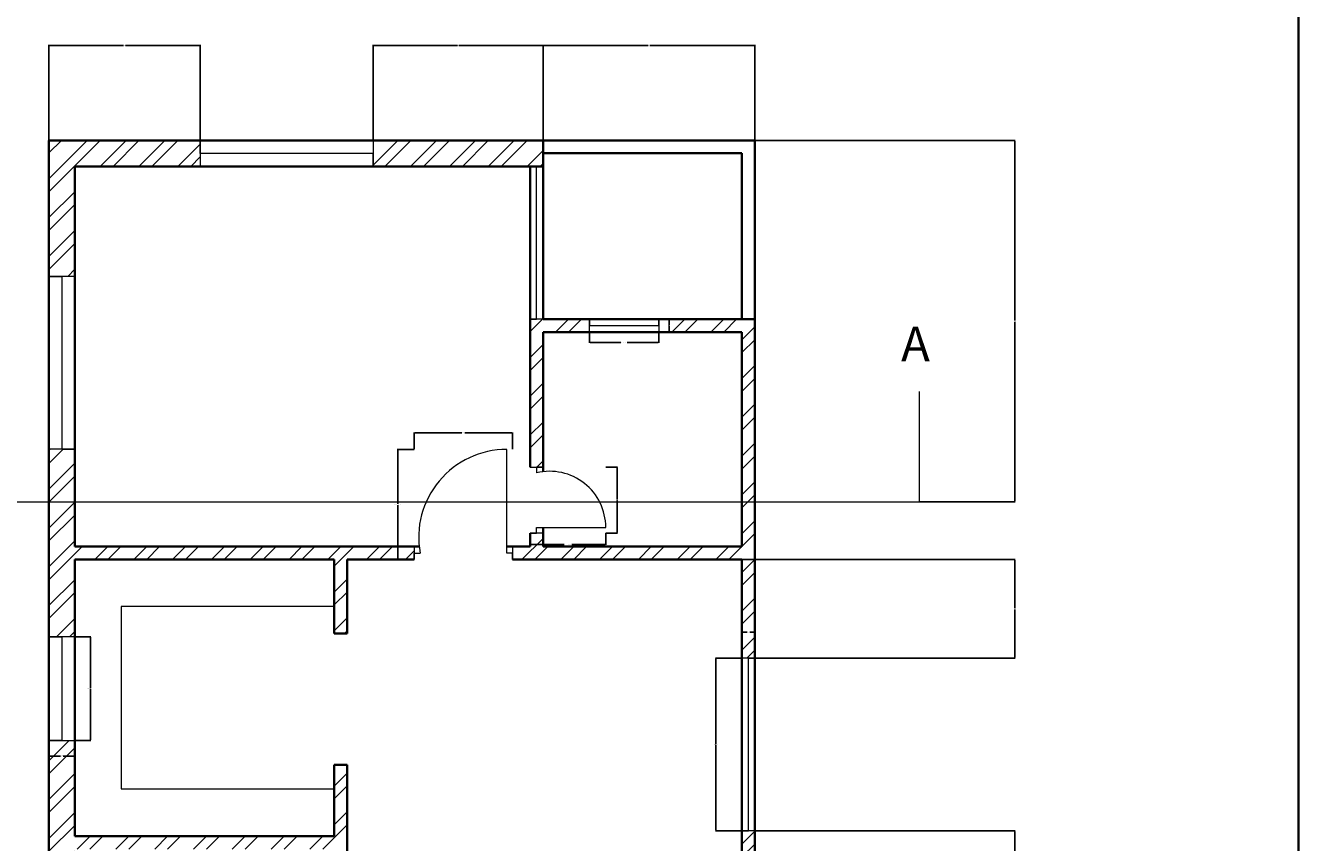
# Model space of a CAD drawing. Units: inches. Extents: x 1850 to 3445, y 1558 to 2756.
# Tile 12 of 13: x 3003 to 3445, y 1972 to 2256. Entities that reach past the tile are written whole.
import ezdxf

# ---------------------------------------------------------------- set-up
doc = ezdxf.new("R2010")
doc.units = ezdxf.units.IN
for name, color, linetype, lineweight in [('A-ANNO-DIMS', 2, 'Continuous', 18), ('A-ANNO-SYMB', 2, 'Continuous', 18), ('A-ANNO-TTLB', 7, 'Continuous', 35), ('A-DOOR', 3, 'Continuous', 18), ('A-FLOR-CASE', 8, 'Continuous', 18), ('A-GLAZ', 4, 'Continuous', 18), ('A-WALL', 7, 'Continuous', 35), ('A-WALL-PATT', 252, 'Continuous', 13)]:
    doc.layers.add(name, color=color, linetype=linetype, lineweight=lineweight)
doc.styles.get("Standard").update_dxf_attribs({"font": 'arial.ttf'})
doc.dimstyles.get("Standard").update_dxf_attribs({"dimtxt": 0.18, "dimasz": 0.18, "dimexe": 0.18, "dimexo": 0.0625, "dimgap": 0.09, "dimtad": 0, "dimtih": 1, "dimtoh": 1, "dimdec": 4, "dimzin": 0, "dimdsep": 46, "dimtxsty": 'Standard', "dimcen": 0.09, "dimadec": 0, "dimazin": 0, "dimtfac": 1, "dimtdec": 4, "dimtofl": 0, "dimtmove": 0, "dimatfit": 3, "dimfxl": 1, "dimtolj": 1, "dimtzin": 0, "dimarcsym": 0})
pattern_1 = [(45, (660.551, 0), (-6.735192, 6.735192), []), (45, (665.041, 0), (-6.735192, 6.735192), [])]

# ---------------------------------------------------------------- blocks, each defined once
blk = doc.blocks.new('WIN-60-W9')
for p, q in [((0, 9), (0, 0)), ((60, 4.5), (60, 9)), ((60, 9), (60, 0)), ((0, 0), (0, 4.5)), ((0, 4.5), (60, 4.5))]:
    blk.add_line(p, q)
blk = doc.blocks.new('WIN-36-W9-ALT')
for p, q in [((9, 36), (0, 36)), ((0, 36), (4.5, 36)), ((4.5, 36), (4.5, 0)), ((4.5, 0), (0, 0)), ((0, 0), (9, 0))]:
    blk.add_line(p, q)
blk = doc.blocks.new('WIN-60-W4_5')
for p, q in [((0, 60), (4.5, 60)), ((4.5, 60), (2.25, 60)), ((2.25, 60), (2.25, 0)), ((2.25, 0), (0, 0)), ((0, 0), (4.5, 0))]:
    blk.add_line(p, q)
blk = doc.blocks.new('WIN-24-W4_5')
for p, q in [((0, 0), (0, 4.5)), ((0, 4.5), (0, 2.25)), ((24, 2.25), (24, 4.5)), ((24, 4.5), (24, 0)), ((0, 2.25), (24, 2.25))]:
    blk.add_line(p, q)
blk = doc.blocks.new('DOOR-BATH-REAR-UPPER')
for p, q in [((0, 22.93), (4.5, 22.93)), ((4.5, 22.93), (2.25, 22.93)), ((2.25, 22.93), (2.25, 20.93)), ((2.25, 0), (2.25, 2)), ((2.25, 2), (26.25, 2)), ((4.5, 0), (0, 0)), ((0, 0), (2.25, 0))]:
    blk.add_line(p, q)
blk.add_arc((6.78, 2), 19.47, 0, 103.4712)
blk = doc.blocks.new('DOOR-BED-UPPER')
for p, q in [((32.07, 2.25), (32.07, 38.25)), ((0, 4.5), (0, 0)), ((34.07, 4.5), (34.07, 0)), ((0, 0), (0, 2.25)), ((0, 2.25), (2, 2.25)), ((34.07, 2.25), (32.07, 2.25)), ((34.07, 0), (34.07, 2.25))]:
    blk.add_line(p, q)
blk.add_arc((32.07, 7.69), 30.56, 90, 190.2532)
blk = doc.blocks.new('COUNTER-U-UPPER')
for p, q in [((73.88, 63.24), (0, 63.24)), ((0, 63.24), (0, 0)), ((0, 0), (73.88, 0))]:
    blk.add_line(p, q)
blk = doc.blocks.new('*D30')
at = {"layer": 'A-ANNO-DIMS', "color": 0, "lineweight": -2, "transparency": 16777216}
for p, q in [((3252.04, 2036.5), (3242.93, 2036.5)), ((3243.11, 2036.32), (3243.11, 2006.68)), ((3243.11, 1976.68), (3243.11, 2006.31)), ((3252.04, 1976.5), (3242.93, 1976.5))]:
    blk.add_line(p, q, dxfattribs=at)
at = {"layer": 'A-ANNO-DIMS', "color": 0, "transparency": 16777216}
for points in [[(3243.08, 2036.32), (3243.14, 2036.32), (3243.11, 2036.5)], [(3243.08, 1976.68), (3243.14, 1976.68), (3243.11, 1976.5)]]:
    blk.add_solid(points, dxfattribs=at)
at = {"layer": 'Defpoints', "color": 0, "transparency": 16777216}
for p in [(3252.11, 2036.5), (3243.11, 1976.5), (3252.11, 1976.5)]:
    blk.add_point(p, dxfattribs=at)
at = {"layer": 'A-ANNO-DIMS', "color": 0, "transparency": 16777216, "insert": (3243.11, 2006.5), "char_height": 0.18, "attachment_point": 5}
blk.add_mtext('\\A1;WINDOW 60 TYP.', dxfattribs=at)
blk = doc.blocks.new('*D31')
at = {"layer": 'A-ANNO-DIMS', "color": 0, "lineweight": -2, "transparency": 16777216}
for p, q in [((3252.11, 2036.56), (3252.11, 2045.68)), ((3256.61, 2036.56), (3256.61, 2045.68)), ((3252.29, 2045.5), (3253.9, 2045.5)), ((3256.43, 2045.5), (3254.81, 2045.5))]:
    blk.add_line(p, q, dxfattribs=at)
at = {"layer": 'A-ANNO-DIMS', "color": 0, "transparency": 16777216}
for points in [[(3252.29, 2045.53), (3252.29, 2045.47), (3252.11, 2045.5)], [(3256.43, 2045.53), (3256.43, 2045.47), (3256.61, 2045.5)]]:
    blk.add_solid(points, dxfattribs=at)
at = {"layer": 'Defpoints', "color": 0, "transparency": 16777216}
for p in [(3252.11, 2045.5), (3252.11, 2036.5), (3256.61, 2036.5)]:
    blk.add_point(p, dxfattribs=at)
at = {"layer": 'A-ANNO-DIMS', "color": 0, "transparency": 16777216, "insert": (3254.36, 2045.5), "char_height": 0.18, "attachment_point": 5}
blk.add_mtext('\\A1;5 TYP.', dxfattribs=at)
blk = doc.blocks.new('*D38')
at = {"layer": 'A-ANNO-DIMS', "color": 0, "lineweight": -2, "transparency": 16777216}
for p, q in [((3020.67, 2043.87), (3026.19, 2043.87)), ((3026.01, 2043.69), (3026.01, 2026.05)), ((3026.01, 2008.05), (3026.01, 2025.69)), ((3020.67, 2007.87), (3026.19, 2007.87))]:
    blk.add_line(p, q, dxfattribs=at)
at = {"layer": 'A-ANNO-DIMS', "color": 0, "transparency": 16777216}
for points in [[(3025.98, 2043.69), (3026.04, 2043.69), (3026.01, 2043.87)], [(3025.98, 2008.05), (3026.04, 2008.05), (3026.01, 2007.87)]]:
    blk.add_solid(points, dxfattribs=at)
at = {"layer": 'Defpoints', "color": 0, "transparency": 16777216}
for p in [(3020.61, 2043.87), (3026.01, 2043.87), (3020.61, 2007.87)]:
    blk.add_point(p, dxfattribs=at)
at = {"layer": 'A-ANNO-DIMS', "color": 0, "transparency": 16777216, "insert": (3026.01, 2025.87), "char_height": 0.18, "attachment_point": 5}
blk.add_mtext('\\A1;WINDOW 36 TYP.', dxfattribs=at)
blk = doc.blocks.new('*D39')
at = {"layer": 'A-ANNO-DIMS', "color": 0, "lineweight": -2, "transparency": 16777216}
for p, q in [((3011.61, 2007.81), (3011.61, 2002.29)), ((3020.61, 2007.81), (3020.61, 2002.29)), ((3011.79, 2002.47), (3015.65, 2002.47)), ((3020.43, 2002.47), (3016.56, 2002.47))]:
    blk.add_line(p, q, dxfattribs=at)
at = {"layer": 'A-ANNO-DIMS', "color": 0, "transparency": 16777216}
for points in [[(3011.79, 2002.5), (3011.79, 2002.44), (3011.61, 2002.47)], [(3020.43, 2002.5), (3020.43, 2002.44), (3020.61, 2002.47)]]:
    blk.add_solid(points, dxfattribs=at)
at = {"layer": 'Defpoints', "color": 0, "transparency": 16777216}
for p in [(3011.61, 2007.87), (3020.61, 2007.87), (3020.61, 2002.47)]:
    blk.add_point(p, dxfattribs=at)
at = {"layer": 'A-ANNO-DIMS', "color": 0, "transparency": 16777216, "insert": (3016.11, 2002.47), "char_height": 0.18, "attachment_point": 5}
blk.add_mtext('\\A1;9 TYP.', dxfattribs=at)
blk = doc.blocks.new('*D42')
at = {"layer": 'A-ANNO-DIMS', "color": 0, "lineweight": -2, "transparency": 16777216}
for p, q in [((3199.22, 2149.62), (3199.22, 2145.9)), ((3223.22, 2149.62), (3223.22, 2145.9)), ((3199.4, 2146.08), (3210.1, 2146.08)), ((3223.04, 2146.08), (3212.33, 2146.08))]:
    blk.add_line(p, q, dxfattribs=at)
at = {"layer": 'A-ANNO-DIMS', "color": 0, "transparency": 16777216}
for points in [[(3199.4, 2146.11), (3199.4, 2146.05), (3199.22, 2146.08)], [(3223.04, 2146.11), (3223.04, 2146.05), (3223.22, 2146.08)]]:
    blk.add_solid(points, dxfattribs=at)
at = {"layer": 'Defpoints', "color": 0, "transparency": 16777216}
for p in [(3199.22, 2149.68), (3223.22, 2149.68), (3223.22, 2146.08)]:
    blk.add_point(p, dxfattribs=at)
at = {"layer": 'A-ANNO-DIMS', "color": 0, "transparency": 16777216, "insert": (3211.22, 2146.08), "char_height": 0.18, "attachment_point": 5}
blk.add_mtext('\\A1;WINDOW 24 TYP.', dxfattribs=at)
blk = doc.blocks.new('*D43')
at = {"layer": 'A-ANNO-DIMS', "color": 0, "lineweight": -2, "transparency": 16777216}
for p, q in [((3223.28, 2154.18), (3227, 2154.18)), ((3226.82, 2154), (3226.82, 2152.12)), ((3226.82, 2149.86), (3226.82, 2151.75)), ((3223.28, 2149.68), (3227, 2149.68))]:
    blk.add_line(p, q, dxfattribs=at)
at = {"layer": 'A-ANNO-DIMS', "color": 0, "transparency": 16777216}
for points in [[(3226.79, 2154), (3226.85, 2154), (3226.82, 2154.18)], [(3226.79, 2149.86), (3226.85, 2149.86), (3226.82, 2149.68)]]:
    blk.add_solid(points, dxfattribs=at)
at = {"layer": 'Defpoints', "color": 0, "transparency": 16777216}
for p in [(3223.22, 2154.18), (3226.82, 2154.18), (3223.22, 2149.68)]:
    blk.add_point(p, dxfattribs=at)
at = {"layer": 'A-ANNO-DIMS', "color": 0, "transparency": 16777216, "insert": (3226.82, 2151.93), "char_height": 0.18, "attachment_point": 5}
blk.add_mtext('\\A1;5 TYP.', dxfattribs=at)
blk = doc.blocks.new('*D62')
at = {"layer": 'A-ANNO-DIMS', "color": 0, "lineweight": -2, "transparency": 16777216}
for p, q in [((3178.61, 2079.81), (3178.61, 2075.75)), ((3204.86, 2079.81), (3204.86, 2075.75)), ((3178.79, 2075.93), (3190.42, 2075.93)), ((3204.68, 2075.93), (3193.04, 2075.93))]:
    blk.add_line(p, q, dxfattribs=at)
at = {"layer": 'A-ANNO-DIMS', "color": 0, "transparency": 16777216}
for points in [[(3178.79, 2075.96), (3178.79, 2075.9), (3178.61, 2075.93)], [(3204.68, 2075.96), (3204.68, 2075.9), (3204.86, 2075.93)]]:
    blk.add_solid(points, dxfattribs=at)
at = {"layer": 'Defpoints', "color": 0, "transparency": 16777216}
for p in [(3178.61, 2079.87), (3204.86, 2079.87), (3204.86, 2075.93)]:
    blk.add_point(p, dxfattribs=at)
at = {"layer": 'A-ANNO-DIMS', "color": 0, "transparency": 16777216, "insert": (3191.73, 2075.93), "char_height": 0.18, "attachment_point": 5}
blk.add_mtext('\\A1;BATH DOOR 26 TYP.', dxfattribs=at)
blk = doc.blocks.new('*D63')
at = {"layer": 'A-ANNO-DIMS', "color": 0, "lineweight": -2, "transparency": 16777216}
for p, q in [((3204.92, 2102.8), (3208.97, 2102.8)), ((3208.79, 2102.62), (3208.79, 2091.52)), ((3208.79, 2080.05), (3208.79, 2091.15)), ((3204.92, 2079.87), (3208.97, 2079.87))]:
    blk.add_line(p, q, dxfattribs=at)
at = {"layer": 'A-ANNO-DIMS', "color": 0, "transparency": 16777216}
for points in [[(3208.76, 2102.62), (3208.82, 2102.62), (3208.79, 2102.8)], [(3208.76, 2080.05), (3208.82, 2080.05), (3208.79, 2079.87)]]:
    blk.add_solid(points, dxfattribs=at)
at = {"layer": 'Defpoints', "color": 0, "transparency": 16777216}
for p in [(3204.86, 2102.8), (3208.79, 2102.8), (3204.86, 2079.87)]:
    blk.add_point(p, dxfattribs=at)
at = {"layer": 'A-ANNO-DIMS', "color": 0, "transparency": 16777216, "insert": (3208.79, 2091.33), "char_height": 0.18, "attachment_point": 5}
blk.add_mtext('\\A1;23 TYP.', dxfattribs=at)
blk = doc.blocks.new('*D64')
at = {"layer": 'A-ANNO-DIMS', "color": 0, "lineweight": -2, "transparency": 16777216}
for p, q in [((3138.36, 2108.93), (3132.5, 2108.93)), ((3132.68, 2108.75), (3132.68, 2089.99)), ((3132.68, 2070.86), (3132.68, 2089.63)), ((3138.36, 2070.68), (3132.5, 2070.68))]:
    blk.add_line(p, q, dxfattribs=at)
at = {"layer": 'A-ANNO-DIMS', "color": 0, "transparency": 16777216}
for points in [[(3132.65, 2108.75), (3132.71, 2108.75), (3132.68, 2108.93)], [(3132.65, 2070.86), (3132.71, 2070.86), (3132.68, 2070.68)]]:
    blk.add_solid(points, dxfattribs=at)
at = {"layer": 'Defpoints', "color": 0, "transparency": 16777216}
for p in [(3132.68, 2108.93), (3138.42, 2108.93), (3138.42, 2070.68)]:
    blk.add_point(p, dxfattribs=at)
at = {"layer": 'A-ANNO-DIMS', "color": 0, "transparency": 16777216, "insert": (3132.68, 2089.81), "char_height": 0.18, "attachment_point": 5}
blk.add_mtext('\\A1;BED DOOR 38 TYP.', dxfattribs=at)
blk = doc.blocks.new('*D65')
at = {"layer": 'A-ANNO-DIMS', "color": 0, "lineweight": -2, "transparency": 16777216}
for p, q in [((3138.42, 2109), (3138.42, 2114.85)), ((3138.6, 2114.67), (3154.93, 2114.67)), ((3172.31, 2114.67), (3155.98, 2114.67)), ((3172.49, 2109), (3172.49, 2114.85))]:
    blk.add_line(p, q, dxfattribs=at)
at = {"layer": 'A-ANNO-DIMS', "color": 0, "transparency": 16777216}
for points in [[(3138.6, 2114.7), (3138.6, 2114.64), (3138.42, 2114.67)], [(3172.31, 2114.7), (3172.31, 2114.64), (3172.49, 2114.67)]]:
    blk.add_solid(points, dxfattribs=at)
at = {"layer": 'Defpoints', "color": 0, "transparency": 16777216}
for p in [(3172.49, 2114.67), (3138.42, 2108.93), (3172.49, 2108.93)]:
    blk.add_point(p, dxfattribs=at)
at = {"layer": 'A-ANNO-DIMS', "color": 0, "transparency": 16777216, "insert": (3155.46, 2114.67), "char_height": 0.18, "attachment_point": 5}
blk.add_mtext('\\A1;34 TYP.', dxfattribs=at)
blk = doc.blocks.new('*D85')
at = {"layer": 'A-ANNO-DIMS', "color": 0, "lineweight": -2, "transparency": 16777216}
for p, q in [((3256.67, 2216.18), (3346.97, 2216.18)), ((3346.79, 2216), (3346.79, 2153.65)), ((3346.79, 2090.94), (3346.79, 2153.29)), ((3313.8, 2090.76), (3346.97, 2090.76))]:
    blk.add_line(p, q, dxfattribs=at)
at = {"layer": 'A-ANNO-DIMS', "color": 0, "transparency": 16777216}
for points in [[(3346.76, 2216), (3346.82, 2216), (3346.79, 2216.18)], [(3346.76, 2090.94), (3346.82, 2090.94), (3346.79, 2090.76)]]:
    blk.add_solid(points, dxfattribs=at)
at = {"layer": 'Defpoints', "color": 0, "transparency": 16777216}
for p in [(3256.61, 2216.18), (3313.74, 2090.76), (3346.79, 2090.76)]:
    blk.add_point(p, dxfattribs=at)
at = {"layer": 'A-ANNO-DIMS', "color": 0, "transparency": 16777216, "insert": (3346.79, 2153.47), "char_height": 0.18, "attachment_point": 5}
blk.add_mtext('\\A1;125.42', dxfattribs=at)
blk = doc.blocks.new('*D89')
at = {"layer": 'A-ANNO-DIMS', "color": 0, "lineweight": -2, "transparency": 16777216}
for p, q in [((3011.61, 2216.25), (3011.61, 2249.41)), ((3011.79, 2249.23), (3037.53, 2249.23)), ((3063.93, 2249.23), (3038.18, 2249.23)), ((3064.11, 2216.25), (3064.11, 2249.41))]:
    blk.add_line(p, q, dxfattribs=at)
at = {"layer": 'A-ANNO-DIMS', "color": 0, "transparency": 16777216}
for points in [[(3011.79, 2249.26), (3011.79, 2249.2), (3011.61, 2249.23)], [(3063.93, 2249.26), (3063.93, 2249.2), (3064.11, 2249.23)]]:
    blk.add_solid(points, dxfattribs=at)
at = {"layer": 'Defpoints', "color": 0, "transparency": 16777216}
for p in [(3064.11, 2249.23), (3011.61, 2216.18), (3064.11, 2216.18)]:
    blk.add_point(p, dxfattribs=at)
at = {"layer": 'A-ANNO-DIMS', "color": 0, "transparency": 16777216, "insert": (3037.86, 2249.23), "char_height": 0.18, "attachment_point": 5}
blk.add_mtext('\\A1;52.5', dxfattribs=at)
blk = doc.blocks.new('*D90')
at = {"layer": 'A-ANNO-DIMS', "color": 0, "lineweight": -2, "transparency": 16777216}
for p, q in [((3124.11, 2216.25), (3124.11, 2249.41)), ((3124.29, 2249.23), (3153.39, 2249.23)), ((3182.93, 2249.23), (3153.83, 2249.23)), ((3183.11, 2216.25), (3183.11, 2249.41))]:
    blk.add_line(p, q, dxfattribs=at)
at = {"layer": 'A-ANNO-DIMS', "color": 0, "transparency": 16777216}
for points in [[(3124.29, 2249.26), (3124.29, 2249.2), (3124.11, 2249.23)], [(3182.93, 2249.26), (3182.93, 2249.2), (3183.11, 2249.23)]]:
    blk.add_solid(points, dxfattribs=at)
at = {"layer": 'Defpoints', "color": 0, "transparency": 16777216}
for p in [(3183.11, 2249.23), (3124.11, 2216.18), (3183.11, 2216.18)]:
    blk.add_point(p, dxfattribs=at)
at = {"layer": 'A-ANNO-DIMS', "color": 0, "transparency": 16777216, "insert": (3153.61, 2249.23), "char_height": 0.18, "attachment_point": 5}
blk.add_mtext('\\A1;59', dxfattribs=at)
blk = doc.blocks.new('*D91')
at = {"layer": 'A-ANNO-DIMS', "color": 0, "lineweight": -2, "transparency": 16777216}
for p, q in [((3183.11, 2216.25), (3183.11, 2249.41)), ((3183.29, 2249.23), (3219.53, 2249.23)), ((3256.43, 2249.23), (3220.18, 2249.23)), ((3256.61, 2216.25), (3256.61, 2249.41))]:
    blk.add_line(p, q, dxfattribs=at)
at = {"layer": 'A-ANNO-DIMS', "color": 0, "transparency": 16777216}
for points in [[(3183.29, 2249.26), (3183.29, 2249.2), (3183.11, 2249.23)], [(3256.43, 2249.26), (3256.43, 2249.2), (3256.61, 2249.23)]]:
    blk.add_solid(points, dxfattribs=at)
at = {"layer": 'Defpoints', "color": 0, "transparency": 16777216}
for p in [(3256.61, 2249.23), (3183.11, 2216.18), (3256.61, 2216.18)]:
    blk.add_point(p, dxfattribs=at)
at = {"layer": 'A-ANNO-DIMS', "color": 0, "transparency": 16777216, "insert": (3219.86, 2249.23), "char_height": 0.18, "attachment_point": 5}
blk.add_mtext('\\A1;73.5', dxfattribs=at)
blk = doc.blocks.new('*D104')
at = {"layer": 'A-ANNO-DIMS', "color": 0, "lineweight": -2, "transparency": 16777216}
for p, q in [((3256.67, 1976.5), (3346.97, 1976.5)), ((3346.79, 1976.32), (3346.79, 1942.13)), ((3346.79, 1907.57), (3346.79, 1941.76)), ((3252.17, 1907.39), (3346.97, 1907.39))]:
    blk.add_line(p, q, dxfattribs=at)
at = {"layer": 'A-ANNO-DIMS', "color": 0, "transparency": 16777216}
for points in [[(3346.76, 1976.32), (3346.82, 1976.32), (3346.79, 1976.5)], [(3346.76, 1907.57), (3346.82, 1907.57), (3346.79, 1907.39)]]:
    blk.add_solid(points, dxfattribs=at)
at = {"layer": 'Defpoints', "color": 0, "transparency": 16777216}
for p in [(3256.61, 1976.5), (3346.79, 1976.5), (3252.11, 1907.39)]:
    blk.add_point(p, dxfattribs=at)
at = {"layer": 'A-ANNO-DIMS', "color": 0, "transparency": 16777216, "insert": (3346.79, 1941.94), "char_height": 0.18, "attachment_point": 5}
blk.add_mtext('\\A1;69.1', dxfattribs=at)
blk = doc.blocks.new('*D105')
at = {"layer": 'A-ANNO-DIMS', "color": 0, "lineweight": -2, "transparency": 16777216}
for p, q in [((3252.17, 2070.68), (3346.97, 2070.68)), ((3346.79, 2070.5), (3346.79, 2053.77)), ((3346.79, 2036.68), (3346.79, 2053.41)), ((3256.67, 2036.5), (3346.97, 2036.5))]:
    blk.add_line(p, q, dxfattribs=at)
at = {"layer": 'A-ANNO-DIMS', "color": 0, "transparency": 16777216}
for points in [[(3346.76, 2070.5), (3346.82, 2070.5), (3346.79, 2070.68)], [(3346.76, 2036.68), (3346.82, 2036.68), (3346.79, 2036.5)]]:
    blk.add_solid(points, dxfattribs=at)
at = {"layer": 'Defpoints', "color": 0, "transparency": 16777216}
for p in [(3252.11, 2070.68), (3346.79, 2070.68), (3256.61, 2036.5)]:
    blk.add_point(p, dxfattribs=at)
at = {"layer": 'A-ANNO-DIMS', "color": 0, "transparency": 16777216, "insert": (3346.79, 2053.59), "char_height": 0.18, "attachment_point": 5}
blk.add_mtext('\\A1;34.19', dxfattribs=at)

msp = doc.modelspace()

# ---------------------------------------------------------------- hatches: boundary and pattern name
at = {"layer": 'A-WALL-PATT'}
h = msp.add_hatch(dxfattribs=at)
h.set_pattern_fill('ANSI32', color=256)
h.set_pattern_definition(pattern_1)
h.paths.add_polyline_path([(3180.1061, 1907.3936), (3184.5492, 1907.3936), (3184.5492, 1916.3936), (3180.1061, 1916.3936), (3175.6061, 1916.3936), (3171.1061, 1916.3936), (3171.1061, 1907.3936), (3175.6061, 1907.3936), (3175.6061, 1742.1843), (3175.6061, 1737.6843), (3256.6061, 1737.6843), (3256.6061, 1976.4962), (3252.1061, 1976.4962), (3252.1061, 1916.3936), (3221.8172, 1916.3936), (3221.8172, 1907.3936), (3252.1061, 1907.3936), (3252.1061, 1746.6843), (3180.1061, 1746.6843)])
h.paths.add_polyline_path([(2737.1986, 2211.6843), (2737.1986, 2216.1843), (2700.822, 2216.1843), (2700.822, 2175.83), (2705.322, 2175.83), (2709.822, 2175.83), (2709.822, 2207.1843), (2737.1986, 2207.1843)])
h.paths.add_polyline_path([(2872.322, 2216.1843), (2797.1986, 2216.1843), (2797.1986, 2207.1843), (2872.322, 2207.1843)])
h.paths.add_polyline_path([(2945.822, 2154.1843), (2911.1674, 2154.1843), (2911.1674, 2149.6843), (2941.322, 2149.6843), (2941.322, 2075.1843), (2896.9138, 2075.1843), (2896.9138, 2070.6843), (2945.822, 2070.6843)])
h.paths.add_polyline_path([(2888.8991, 2154.1843), (2867.822, 2154.1843), (2867.822, 2075.1843), (2862.5325, 2075.1843), (2862.5325, 2070.6843), (2876.0169, 2070.6843), (2876.0169, 2072.9343), (2876.0169, 2075.1843), (2872.322, 2075.1843), (2872.322, 2149.6843), (2888.8991, 2149.6843)])
h.paths.add_polyline_path([(2709.822, 2115.83), (2700.822, 2115.83), (2700.822, 2042.8465), (2709.822, 2042.8465), (2709.822, 2070.6843), (2829.1562, 2070.6843), (2829.1562, 2072.9343), (2829.1562, 2075.1843), (2709.822, 2075.1843)])
h.paths.add_polyline_path([(2709.822, 1982.8465), (2700.822, 1982.8465), (2700.822, 1910.2175), (2721.4986, 1910.2175), (2721.4986, 1914.7175), (2721.4986, 1919.2175), (2709.822, 1919.2175)])
h.paths.add_polyline_path([(2793.0443, 1919.2175), (2769.4986, 1919.2175), (2769.4986, 1910.2175), (2793.0443, 1910.2175), (2793.0443, 1914.6749)])
h.paths.add_polyline_path([(2839.322, 1938.6843), (2830.322, 1938.6843), (2830.322, 1919.2175), (2824.2376, 1919.2175), (2824.2376, 1910.2175), (2830.322, 1910.2175), (2830.322, 1854.6843), (2830.322, 1845.6843), (2856.6792, 1845.6843), (2856.6792, 1850.1843), (2856.6792, 1854.6843), (2839.322, 1854.6843)])
h.paths.add_polyline_path([(2709.822, 1910.2175), (2700.822, 1910.2175), (2700.822, 1745.6843), (2709.822, 1745.6843)])
h.paths.add_polyline_path([(2807.4367, 1766.7204), (2819.64, 1766.7204), (2819.64, 1777.0239), (2807.4367, 1777.0239)], flags=9)
h.paths.add_polyline_path([(2844.0169, 1798.4016), (2887.2843, 1798.4016), (2887.2843, 1817.0589), (2844.0169, 1817.0589)], flags=9)
h.paths.add_polyline_path([(2731.4135, 1867.537), (2770.5302, 1867.537), (2770.5302, 1886.1943), (2731.4135, 1886.1943)], flags=9)
h = msp.add_hatch(dxfattribs=at)
h.set_pattern_fill('ANSI32', color=256)
h.set_pattern_definition(pattern_1)
h.paths.add_polyline_path([(3064.1082, 2211.6843), (3064.1082, 2216.1843), (3011.6061, 2216.1843), (3011.6061, 2169.0079), (3020.6061, 2169.0079), (3020.6061, 2207.1843), (3064.1082, 2207.1843)])
h.paths.add_polyline_path([(3183.1061, 2216.1843), (3124.1082, 2216.1843), (3124.1082, 2207.1843), (3183.1061, 2207.1843)])
h.paths.add_polyline_path([(3256.6061, 2154.1843), (3223.2152, 2154.1843), (3223.2152, 2149.6843), (3252.1061, 2149.6843), (3252.1061, 2075.1843), (3183.1061, 2075.1843), (3183.1061, 2079.8699), (3178.6061, 2079.8699), (3178.6061, 2075.1843), (3172.4917, 2075.1843), (3172.4917, 2070.6843), (3252.1061, 2070.6843), (3252.1061, 2036.4962), (3256.6061, 2036.4962)])
h.paths.add_polyline_path([(3199.2152, 2154.1843), (3183.1061, 2154.1843), (3178.6061, 2154.1843), (3178.6061, 2102.7998), (3183.1061, 2102.7998), (3183.1061, 2149.6843), (3199.2152, 2149.6843)], flags=17)
h.paths.add_polyline_path([(3138.4194, 2072.9343), (3138.4194, 2075.1843), (3020.6061, 2075.1843), (3020.6061, 2109.0079), (3016.1061, 2109.0079), (3011.6061, 2109.0079), (3011.6061, 2043.8694), (3016.1061, 2043.8694), (3020.6061, 2043.8694), (3020.6061, 2070.6843), (3110.6061, 2070.6843), (3110.6061, 2045.0271), (3115.1061, 2045.0271), (3115.1061, 2070.6843), (3138.4194, 2070.6843)])
h.paths.add_polyline_path([(3020.6061, 2007.8694), (3011.6061, 2007.8694), (3011.6061, 1958.9131), (3016.1061, 1958.9131), (3020.6061, 1958.9131), (3020.6061, 1970.1843), (3110.6061, 1970.1843), (3110.6061, 1913.1843), (3104.2838, 1913.1843), (3104.2838, 1908.6843), (3115.1061, 1908.6843), (3115.1061, 1999.4184), (3110.6061, 1999.4184), (3110.6061, 1974.6843), (3020.6061, 1974.6843)])
h.paths.add_polyline_path([(3020.6061, 1908.6843), (3082.9753, 1908.6843), (3082.9753, 1910.9343), (3082.9753, 1913.1843), (3020.6061, 1913.1843), (3020.6061, 1934.9131), (3011.6061, 1934.9131), (3011.6061, 1778.1843), (3086.5835, 1778.1843), (3086.5835, 1780.4343), (3086.5835, 1782.6843), (3020.6061, 1782.6843)])
h.paths.add_polyline_path([(3175.6061, 1782.6843), (3146.5835, 1782.6843), (3146.5835, 1778.1843), (3175.6061, 1778.1843)])

# ---------------------------------------------------------------- linework, layer by layer
at = {"layer": 'A-ANNO-SYMB'}
for p, q in [((3313.7387, 2090.7612), (3313.7387, 2129.0942)), ((2673.1156, 2090.7612), (3313.7387, 2090.7612))]:
    msp.add_line(p, q, dxfattribs=at)
at = {"layer": 'A-ANNO-TTLB'}
msp.add_lwpolyline([(1850.1793, 2756.3177), (3445.2682, 2756.3177), (3445.2682, 1557.7728), (1850.1793, 1557.7728)], close=True, dxfattribs=at)
at = {"layer": 'A-GLAZ'}
for p, q in [((3180.8561, 2154.1843), (3180.8561, 2207.1843)), ((3183.1061, 2154.1843), (3178.6061, 2154.1843)), ((3178.6061, 2154.1843), (3180.8561, 2154.1843))]:
    msp.add_line(p, q, dxfattribs=at)
at = {"layer": 'A-WALL'}
for p, q in [((3011.6061, 2216.1843), (3256.6061, 2216.1843)), ((3011.6061, 2216.1843), (3011.6061, 1737.6843)), ((3183.1061, 2216.1843), (3183.1061, 2154.1843)), ((3256.6061, 2216.1843), (3256.6061, 1737.6843)), ((3183.1061, 2211.8264), (3252.1061, 2211.8264)), ((3252.1061, 2211.8264), (3252.1061, 2207.1843)), ((3020.6061, 2207.1843), (3183.1061, 2207.1843)), ((3020.6061, 2207.1843), (3020.6061, 2075.1843)), ((3178.6061, 2207.1843), (3178.6061, 2102.7998)), ((3252.1061, 2207.1843), (3252.1061, 2154.1843)), ((3183.1061, 2154.1843), (3256.6061, 2154.1843)), ((3183.1061, 2149.6843), (3252.1061, 2149.6843)), ((3183.1061, 2149.6843), (3183.1061, 2101.2008)), ((3252.1061, 2149.6843), (3252.1061, 2075.1843)), ((3183.1061, 2081.8699), (3183.1061, 2075.1843)), ((3178.6061, 2079.8699), (3178.6061, 2075.1843)), ((3020.6061, 2075.1843), (3140.0983, 2075.1843)), ((3170.4917, 2075.1843), (3178.6061, 2075.1843)), ((3183.1061, 2075.1843), (3252.1061, 2075.1843)), ((3020.6061, 2070.6843), (3110.6061, 2070.6843)), ((3020.6061, 2070.6843), (3020.6061, 1974.6843)), ((3110.6061, 2070.6843), (3110.6061, 2045.0271)), ((3115.1061, 2070.6843), (3138.4194, 2070.6843)), ((3115.1061, 2070.6843), (3115.1061, 2045.0271)), ((3172.4917, 2070.6843), (3252.1061, 2070.6843)), ((3252.1061, 2070.6843), (3252.1061, 1916.3936)), ((3110.6061, 2045.0271), (3115.1061, 2045.0271)), ((3110.6061, 1999.4184), (3110.6061, 1974.6843)), ((3110.6061, 1999.4184), (3115.1061, 1999.4184)), ((3115.1061, 1999.4184), (3115.1061, 1908.6843)), ((3020.6061, 1974.6843), (3110.6061, 1974.6843))]:
    msp.add_line(p, q, dxfattribs=at)

# ---------------------------------------------------------------- block references
at = {"layer": 'A-DOOR'}
for name, p in [('DOOR-BED-UPPER', (3138.4195, 2070.684)), ('DOOR-BATH-REAR-UPPER', (3178.6065, 2079.87))]:
    msp.add_blockref(name, p, dxfattribs=at)
at = {"layer": 'A-FLOR-CASE'}
msp.add_blockref('COUNTER-U-UPPER', (3036.7295, 1991.114), dxfattribs=at)
at = {"layer": 'A-GLAZ', "extrusion": (0, 0, -1), "zscale": -1}
msp.add_blockref('WIN-60-W9', (-3124.1082, 2207.184), dxfattribs=at)
at = {"layer": 'A-GLAZ'}
for name, p, rotation in [('WIN-60-W9', (3011.6058, 2169.008), 270), ('WIN-60-W4_5', (3256.6066, 2036.4962), 180)]:
    msp.add_blockref(name, p, dxfattribs=dict(at, rotation=rotation))
for name, p in [('WIN-24-W4_5', (3199.2155, 2149.684)), ('WIN-36-W9-ALT', (3011.6065, 2007.869))]:
    msp.add_blockref(name, p, dxfattribs=at)

# ---------------------------------------------------------------- texts
at = {"layer": 'A-ANNO-SYMB', "insert": (3307.3575, 2151.5737), "char_height": 12, "attachment_point": 1}
msp.add_mtext_dynamic_manual_height_columns('A', width=44.593052, gutter_width=12.5, heights=[0], dxfattribs=at)

# ---------------------------------------------------------------- dimensions: what is measured, and where the dimension line sits
at = {"layer": 'A-ANNO-DIMS'}
for base, p1, p2, override, picture, middle in [((3064.1082, 2249.2343), (3011.6061, 2216.1843), (3064.1082, 2216.1843), {"dimdec": 1, "dimlfac": 1, "dimrnd": 0, "dimzin": 0, "dimdsep": 46, "dimlunit": 2}, '*D89', (3037.8571, 2249.2343)), ((3183.1061, 2249.2343), (3124.1082, 2216.1843), (3183.1061, 2216.1843), {"dimdec": 0, "dimlfac": 1, "dimrnd": 0, "dimzin": 0, "dimdsep": 46, "dimlunit": 2}, '*D90', (3153.6071, 2249.2343)), ((3256.6061, 2249.2343), (3183.1061, 2216.1843), (3256.6061, 2216.1843), {"dimdec": 1, "dimlfac": 1, "dimrnd": 0, "dimzin": 0, "dimdsep": 46, "dimlunit": 2}, '*D91', (3219.8561, 2249.2343))]:
    dim = msp.add_linear_dim(base=base, p1=p1, p2=p2, dimstyle='Standard', override=override, dxfattribs=at)
    dim.commit()
    dim.dimension.update_dxf_attribs({"geometry": picture, "text_midpoint": middle})
for base, p1, p2, override, picture, middle in [((3346.7887, 2090.7612), (3256.6061, 2216.1843), (3313.7387, 2090.7612), {"dimdec": 2, "dimlfac": 1, "dimrnd": 0, "dimzin": 0, "dimdsep": 46, "dimlunit": 2}, '*D85', (3346.7887, 2153.4728)), ((3346.7887, 2070.6843), (3256.6061, 2036.4962), (3252.1061, 2070.6843), {"dimdec": 2, "dimlfac": 1, "dimrnd": 0, "dimzin": 0, "dimdsep": 46, "dimlunit": 2}, '*D105', (3346.7887, 2053.5903)), ((3346.7887, 1976.4962), (3252.1061, 1907.3936), (3256.6061, 1976.4962), {"dimdec": 1, "dimlfac": 1, "dimrnd": 0, "dimzin": 0, "dimdsep": 46, "dimlunit": 2}, '*D104', (3346.7887, 1941.9449))]:
    dim = msp.add_linear_dim(base=base, p1=p1, p2=p2, angle=90, dimstyle='Standard', override=override, dxfattribs=at)
    dim.commit()
    dim.dimension.update_dxf_attribs({"geometry": picture, "text_midpoint": middle})
for base, p1, p2, angle, text, picture, middle in [((3226.8152432889, 2154.1842850418), (3223.2152432889, 2149.6842850418), (3223.2152432889, 2154.1842850418), 90, '<> TYP.', '*D43', (3226.8152432889, 2151.9342850418)), ((3132.6819, 2108.9343), (3138.4194, 2070.6843), (3138.4194, 2108.9343), 90, 'BED DOOR <> TYP.', '*D64', (3132.6819, 2089.8093)), ((3208.7936, 2102.7998), (3204.8561, 2079.8699), (3204.8561, 2102.7998), 90, '<> TYP.', '*D63', (3208.7936, 2091.3349)), ((3252.1061198639, 2045.4962159111), (3256.6061198639, 2036.4962159111), (3252.1061198639, 2036.4962159111), 180, '<> TYP.', '*D31', (3254.3561198639, 2045.4962159111)), ((3026.0061, 2043.8694), (3020.6061, 2007.8694), (3020.6061, 2043.8694), 90, 'WINDOW <> TYP.', '*D38', (3026.0061, 2025.8694)), ((3243.1061, 1976.4962), (3252.1061, 2036.4962), (3252.1061, 1976.4962), 270, 'WINDOW <> TYP.', '*D30', (3243.1061, 2006.4962))]:
    dim = msp.add_linear_dim(base=base, p1=p1, p2=p2, angle=angle, text=text, dimstyle='Standard', override={"dimdec": 0, "dimlfac": 1, "dimrnd": 0, "dimzin": 0, "dimdsep": 46, "dimlunit": 2}, dxfattribs=at)
    dim.commit()
    dim.dimension.update_dxf_attribs({"geometry": picture, "text_midpoint": middle})
for base, p1, p2, text, picture, middle in [((3223.2152, 2146.0843), (3199.2152, 2149.6843), (3223.2152, 2149.6843), 'WINDOW <> TYP.', '*D42', (3211.2152, 2146.0843)), ((3172.4917, 2114.6718), (3138.4194, 2108.9343), (3172.4917, 2108.9343), '<> TYP.', '*D65', (3155.4556, 2114.6718)), ((3204.8561, 2075.9324), (3178.6061, 2079.8699), (3204.8561, 2079.8699), 'BATH DOOR <> TYP.', '*D62', (3191.7311, 2075.9324)), ((3020.6061, 2002.4694), (3011.6061, 2007.8694), (3020.6061, 2007.8694), '<> TYP.', '*D39', (3016.1061, 2002.4694))]:
    dim = msp.add_linear_dim(base=base, p1=p1, p2=p2, text=text, dimstyle='Standard', override={"dimdec": 0, "dimlfac": 1, "dimrnd": 0, "dimzin": 0, "dimdsep": 46, "dimlunit": 2}, dxfattribs=at)
    dim.commit()
    dim.dimension.update_dxf_attribs({"geometry": picture, "text_midpoint": middle})

doc.saveas('drawing.dxf')
